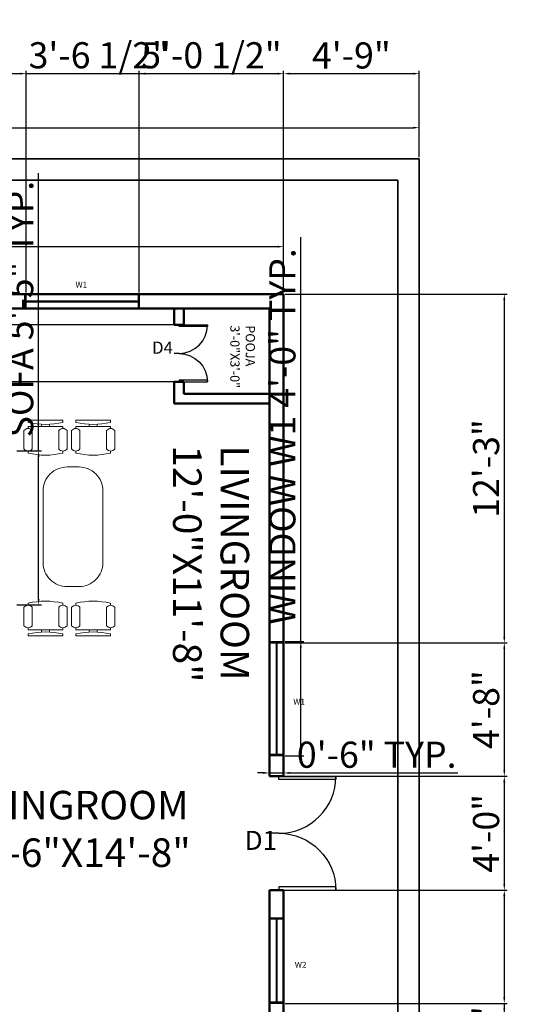
# Model space of a CAD drawing. Units: inches. Extents: x 2299 to 4423, y 1066 to 1805.
# Tile 3 of 7: x 2670 to 2884, y 1391 to 1805. Entities that reach past the tile are written whole.
import ezdxf

# ---------------------------------------------------------------- set-up
doc = ezdxf.new("R2010")
doc.units = ezdxf.units.IN
for name, color, linetype, lineweight in [('A-ANNO-DIMS', 2, 'Continuous', 18), ('A-ANNO-TEXT', 1, 'Continuous', 25), ('A-AREA-IDEN', 1, 'Continuous', 25), ('A-DOOR', 5, 'Continuous', 25), ('A-FURN', 8, 'Continuous', 18), ('A-GLAZ', 3, 'Continuous', 25), ('A-WALL', 7, 'Continuous', 50), ('C-PROP', 7, 'Continuous', 35)]:
    doc.layers.add(name, color=color, linetype=linetype, lineweight=lineweight)
doc.styles.get("Standard").update_dxf_attribs({"font": 'arial.ttf'})
doc.dimstyles.new('ISO-25', dxfattribs={"dimtxt": 11, "dimasz": 2.5, "dimexe": 1.25, "dimexo": 0.625, "dimtad": 1, "dimlunit": 4, "dimtxsty": 'Standard', "dimcen": 2.5, "dimadec": 0, "dimazin": 0, "dimtfac": 1, "dimtmove": 0, "dimatfit": 3, "dimfxl": 1, "dimarcsym": 0})

# ---------------------------------------------------------------- blocks, each defined once
blk = doc.blocks.new('*U2')
for p, q in [((0, 0), (0, -5)), ((30, 0), (30, -5))]:
    blk.add_line(p, q)
blk.add_lwpolyline([(0, 0), (0, 30), (1.75, 30), (1.75, 0)], close=True)
blk.add_arc((0, 0), 30, 0, 90)
blk = doc.blocks.new('Chair - Desk')
for p, q in [((-8.5, 0), (-8.5, -1)), ((-8.5, 0), (8.5, 0)), ((8.5, 0), (8.5, -1)), ((-8.5, -3), (-8.5, -4)), ((-8.5, -3), (8.5, -3)), ((-2, -3), (-2, -1.9355)), ((2, -1.9576), (2, -3)), ((8.5, -3), (8.5, -4)), ((-10.5, -5), (-10.5, -14)), ((-6.5, -14), (-6.5, -5)), ((6.5, -5), (6.5, -14)), ((10.5, -14), (10.5, -5)), ((-8.5, -15), (-8.5, -16)), ((8.5, -15), (8.5, -16))]:
    blk.add_line(p, q)
for centre, radius, start, end in [((-8.5, -6.5), 2.5, 36.8699, 143.1301), ((0, 34.625), 36.625, 256.5803, 283.4197), ((8.5, -6.5), 2.5, 36.8699, 143.1301), ((-8.5, -12.5), 2.5, 216.8699, 323.1301), ((8.5, -12.5), 2.5, 216.8699, 323.1301), ((0, 19.625), 36.625, 256.5803, 283.4197)]:
    blk.add_arc(centre, radius, start, end)
blk = doc.blocks.new('*D20')
at = {"layer": 'A-ANNO-DIMS', "color": 0, "lineweight": -2, "transparency": 16777216}
for p, q in [((2357.83, 1747.57), (2357.83, 1761.24)), ((2360.33, 1759.99), (2835.33, 1759.99)), ((2837.83, 1747.57), (2837.83, 1761.24))]:
    blk.add_line(p, q, dxfattribs=at)
at = {"layer": 'A-ANNO-DIMS', "color": 0, "transparency": 16777216}
for points in [[(2360.33, 1760.41), (2360.33, 1759.58), (2357.83, 1759.99)], [(2835.33, 1760.41), (2835.33, 1759.58), (2837.83, 1759.99)]]:
    blk.add_solid(points, dxfattribs=at)
at = {"layer": 'Defpoints', "color": 0, "transparency": 16777216}
for p in [(2837.83, 1759.99), (2357.83, 1746.95), (2837.83, 1746.95)]:
    blk.add_point(p, dxfattribs=at)
at = {"layer": 'A-ANNO-DIMS', "color": 0, "transparency": 16777216, "insert": (2597.83, 1766.23), "char_height": 11, "attachment_point": 5}
blk.add_mtext("40'", dxfattribs=at)
blk = doc.blocks.new('*D22')
at = {"layer": 'A-ANNO-DIMS', "color": 0, "lineweight": -2, "transparency": 16777216}
for p, q in [((2414.83, 1690.57), (2414.83, 1711.17)), ((2417.33, 1709.92), (2778.33, 1709.92)), ((2780.83, 1690.57), (2780.83, 1711.17))]:
    blk.add_line(p, q, dxfattribs=at)
at = {"layer": 'A-ANNO-DIMS', "color": 0, "transparency": 16777216}
for points in [[(2417.33, 1710.33), (2417.33, 1709.5), (2414.83, 1709.92)], [(2778.33, 1710.33), (2778.33, 1709.5), (2780.83, 1709.92)]]:
    blk.add_solid(points, dxfattribs=at)
at = {"layer": 'Defpoints', "color": 0, "transparency": 16777216}
for p in [(2780.83, 1709.92), (2414.83, 1689.95), (2780.83, 1689.95)]:
    blk.add_point(p, dxfattribs=at)
at = {"layer": 'A-ANNO-DIMS', "color": 0, "transparency": 16777216, "insert": (2597.83, 1716.16), "char_height": 11, "attachment_point": 5}
blk.add_mtext('30\'-6"', dxfattribs=at)
blk = doc.blocks.new('WIN-1200')
for p, q in [((0, 0), (0, 48.07)), ((0, 48.07), (6, 48.07)), ((0, 47.57), (6, 47.57)), ((2.8, 47.57), (2.8, 0.5)), ((3.2, 47.57), (3.2, 0.5)), ((6, 48.07), (6, 0)), ((6, 0.5), (0, 0.5)), ((6, 0), (0, 0))]:
    blk.add_line(p, q)
blk = doc.blocks.new('WIN-900')
for p, q in [((0, 6), (36.07, 6)), ((0, 0), (0, 6)), ((0.5, 0), (0.5, 6)), ((35.57, 6), (35.57, 0)), ((36.07, 6), (36.07, 0)), ((36.07, 0), (0, 0)), ((0.5, 3.2), (35.57, 3.2)), ((0.5, 2.8), (35.57, 2.8))]:
    blk.add_line(p, q)
blk = doc.blocks.new('*D38')
at = {"layer": 'A-ANNO-DIMS', "color": 0, "lineweight": -2, "transparency": 16777216}
for p, q in [((2788.04, 1543.64), (2788.04, 1713.9)), ((2781.46, 1543.64), (2789.29, 1543.64)), ((2788.04, 1498.07), (2788.04, 1541.14)), ((2781.46, 1495.57), (2789.29, 1495.57))]:
    blk.add_line(p, q, dxfattribs=at)
at = {"layer": 'A-ANNO-DIMS', "color": 0, "transparency": 16777216}
for points in [[(2787.63, 1541.14), (2788.46, 1541.14), (2788.04, 1543.64)], [(2787.63, 1498.07), (2788.46, 1498.07), (2788.04, 1495.57)]]:
    blk.add_solid(points, dxfattribs=at)
at = {"layer": 'Defpoints', "color": 0, "transparency": 16777216}
for p in [(2780.83, 1543.64), (2788.04, 1543.64), (2780.83, 1495.57)]:
    blk.add_point(p, dxfattribs=at)
at = {"layer": 'A-ANNO-DIMS', "color": 0, "transparency": 16777216, "insert": (2781.73, 1630.02), "char_height": 11, "attachment_point": 5, "rotation": 90}
blk.add_mtext('WINDOW W1 4\'-0" TYP.', dxfattribs=at)
blk = doc.blocks.new('*D39')
at = {"layer": 'A-ANNO-DIMS', "color": 0, "lineweight": -2, "transparency": 16777216}
for p, q in [((2774.83, 1494.94), (2774.83, 1487.1)), ((2780.83, 1494.94), (2780.83, 1487.1)), ((2772.33, 1488.35), (2769.83, 1488.35)), ((2774.83, 1488.35), (2780.83, 1488.35)), ((2783.33, 1488.35), (2854.13, 1488.35))]:
    blk.add_line(p, q, dxfattribs=at)
at = {"layer": 'A-ANNO-DIMS', "color": 0, "transparency": 16777216}
for points in [[(2772.33, 1488.77), (2772.33, 1487.94), (2774.83, 1488.35)], [(2783.33, 1488.77), (2783.33, 1487.94), (2780.83, 1488.35)]]:
    blk.add_solid(points, dxfattribs=at)
at = {"layer": 'Defpoints', "color": 0, "transparency": 16777216}
for p in [(2774.83, 1495.57), (2780.83, 1495.57), (2780.83, 1488.35)]:
    blk.add_point(p, dxfattribs=at)
at = {"layer": 'A-ANNO-DIMS', "color": 0, "transparency": 16777216, "insert": (2819.98, 1494.6), "char_height": 11, "attachment_point": 5}
blk.add_mtext('0\'-6" TYP.', dxfattribs=at)
blk = doc.blocks.new('*D52')
at = {"layer": 'A-ANNO-DIMS', "color": 0, "lineweight": -2, "transparency": 16777216}
for p, q in [((2677.79, 1623.96), (2677.79, 1740.82)), ((2668.68, 1623.96), (2679.04, 1623.96)), ((2677.79, 1561.58), (2677.79, 1621.46)), ((2668.68, 1559.08), (2679.04, 1559.08))]:
    blk.add_line(p, q, dxfattribs=at)
at = {"layer": 'A-ANNO-DIMS', "color": 0, "transparency": 16777216}
for points in [[(2677.37, 1621.46), (2678.21, 1621.46), (2677.79, 1623.96)], [(2677.37, 1561.58), (2678.21, 1561.58), (2677.79, 1559.08)]]:
    blk.add_solid(points, dxfattribs=at)
at = {"layer": 'Defpoints', "color": 0, "transparency": 16777216}
for p in [(2668.06, 1623.96), (2677.79, 1623.96), (2668.06, 1559.08)]:
    blk.add_point(p, dxfattribs=at)
at = {"layer": 'A-ANNO-DIMS', "color": 0, "transparency": 16777216, "insert": (2671.47, 1683.64), "char_height": 11, "attachment_point": 5, "rotation": 90}
blk.add_mtext('SOFA 5\'-5" TYP.', dxfattribs=at)
blk = doc.blocks.new('*D67')
at = {"layer": 'A-ANNO-DIMS', "color": 0, "lineweight": -2, "transparency": 16777216}
for p, q in [((2629.83, 1684.57), (2629.83, 1784)), ((2632.33, 1782.75), (2670.06, 1782.75)), ((2672.56, 1690.57), (2672.56, 1784)), ((2672.56, 1782.75), (2731.17, 1782.75))]:
    blk.add_line(p, q, dxfattribs=at)
at = {"layer": 'A-ANNO-DIMS', "color": 0, "transparency": 16777216}
for points in [[(2632.33, 1783.16), (2632.33, 1782.33), (2629.83, 1782.75)], [(2670.06, 1783.16), (2670.06, 1782.33), (2672.56, 1782.75)]]:
    blk.add_solid(points, dxfattribs=at)
at = {"layer": 'Defpoints', "color": 0, "transparency": 16777216}
for p in [(2672.56, 1782.75), (2672.56, 1689.95), (2629.83, 1683.95)]:
    blk.add_point(p, dxfattribs=at)
at = {"layer": 'A-ANNO-DIMS', "color": 0, "transparency": 16777216, "insert": (2703.11, 1789.06), "char_height": 11, "attachment_point": 5}
blk.add_mtext('3\'-6 1/2"', dxfattribs=at)
blk = doc.blocks.new('*D68')
at = {"layer": 'A-ANNO-DIMS', "color": 0, "lineweight": -2, "transparency": 16777216}
for p, q in [((2720.13, 1690.57), (2720.13, 1784)), ((2722.63, 1782.75), (2778.33, 1782.75)), ((2780.83, 1690.57), (2780.83, 1784))]:
    blk.add_line(p, q, dxfattribs=at)
at = {"layer": 'A-ANNO-DIMS', "color": 0, "transparency": 16777216}
for points in [[(2722.63, 1783.16), (2722.63, 1782.33), (2720.13, 1782.75)], [(2778.33, 1783.16), (2778.33, 1782.33), (2780.83, 1782.75)]]:
    blk.add_solid(points, dxfattribs=at)
at = {"layer": 'Defpoints', "color": 0, "transparency": 16777216}
for p in [(2780.83, 1782.75), (2720.13, 1689.95), (2780.83, 1689.95)]:
    blk.add_point(p, dxfattribs=at)
at = {"layer": 'A-ANNO-DIMS', "color": 0, "transparency": 16777216, "insert": (2750.48, 1789.06), "char_height": 11, "attachment_point": 5}
blk.add_mtext('5\'-0 1/2"', dxfattribs=at)
blk = doc.blocks.new('*D69')
at = {"layer": 'A-ANNO-DIMS', "color": 0, "lineweight": -2, "transparency": 16777216}
for p, q in [((2780.83, 1690.57), (2780.83, 1784)), ((2783.33, 1782.75), (2835.33, 1782.75)), ((2837.83, 1747.57), (2837.83, 1784))]:
    blk.add_line(p, q, dxfattribs=at)
at = {"layer": 'A-ANNO-DIMS', "color": 0, "transparency": 16777216}
for points in [[(2783.33, 1783.16), (2783.33, 1782.33), (2780.83, 1782.75)], [(2835.33, 1783.16), (2835.33, 1782.33), (2837.83, 1782.75)]]:
    blk.add_solid(points, dxfattribs=at)
at = {"layer": 'Defpoints', "color": 0, "transparency": 16777216}
for p in [(2837.83, 1782.75), (2837.83, 1746.95), (2780.83, 1689.95)]:
    blk.add_point(p, dxfattribs=at)
at = {"layer": 'A-ANNO-DIMS', "color": 0, "transparency": 16777216, "insert": (2809.33, 1788.99), "char_height": 11, "attachment_point": 5}
blk.add_mtext('4\'-9"', dxfattribs=at)
blk = doc.blocks.new('*D78')
at = {"layer": 'A-ANNO-DIMS', "color": 0, "lineweight": -2, "transparency": 16777216}
for p, q in [((2781.46, 1689.95), (2874.88, 1689.95)), ((2873.63, 1687.45), (2873.63, 1545.64)), ((2781.46, 1543.14), (2874.88, 1543.14))]:
    blk.add_line(p, q, dxfattribs=at)
at = {"layer": 'A-ANNO-DIMS', "color": 0, "transparency": 16777216}
for points in [[(2873.22, 1687.45), (2874.05, 1687.45), (2873.63, 1689.95)], [(2873.22, 1545.64), (2874.05, 1545.64), (2873.63, 1543.14)]]:
    blk.add_solid(points, dxfattribs=at)
at = {"layer": 'Defpoints', "color": 0, "transparency": 16777216}
for p in [(2780.83, 1689.95), (2780.83, 1543.14), (2873.63, 1543.14)]:
    blk.add_point(p, dxfattribs=at)
at = {"layer": 'A-ANNO-DIMS', "color": 0, "transparency": 16777216, "insert": (2867.39, 1616.54), "char_height": 11, "attachment_point": 5, "rotation": 90}
blk.add_mtext('12\'-3"', dxfattribs=at)
blk = doc.blocks.new('*D79')
at = {"layer": 'A-ANNO-DIMS', "color": 0, "lineweight": -2, "transparency": 16777216}
for p, q in [((2781.46, 1543.14), (2874.88, 1543.14)), ((2873.63, 1540.64), (2873.63, 1489.45)), ((2781.46, 1486.95), (2874.88, 1486.95))]:
    blk.add_line(p, q, dxfattribs=at)
at = {"layer": 'A-ANNO-DIMS', "color": 0, "transparency": 16777216}
for points in [[(2873.22, 1540.64), (2874.05, 1540.64), (2873.63, 1543.14)], [(2873.22, 1489.45), (2874.05, 1489.45), (2873.63, 1486.95)]]:
    blk.add_solid(points, dxfattribs=at)
at = {"layer": 'Defpoints', "color": 0, "transparency": 16777216}
for p in [(2780.83, 1543.14), (2780.83, 1486.95), (2873.63, 1486.95)]:
    blk.add_point(p, dxfattribs=at)
at = {"layer": 'A-ANNO-DIMS', "color": 0, "transparency": 16777216, "insert": (2867.39, 1515.04), "char_height": 11, "attachment_point": 5, "rotation": 90}
blk.add_mtext('4\'-8"', dxfattribs=at)
blk = doc.blocks.new('*D80')
at = {"layer": 'A-ANNO-DIMS', "color": 0, "lineweight": -2, "transparency": 16777216}
for p, q in [((2781.46, 1486.95), (2874.88, 1486.95)), ((2873.63, 1484.45), (2873.63, 1441.45)), ((2781.46, 1438.95), (2874.88, 1438.95))]:
    blk.add_line(p, q, dxfattribs=at)
at = {"layer": 'A-ANNO-DIMS', "color": 0, "transparency": 16777216}
for points in [[(2873.22, 1484.45), (2874.05, 1484.45), (2873.63, 1486.95)], [(2873.22, 1441.45), (2874.05, 1441.45), (2873.63, 1438.95)]]:
    blk.add_solid(points, dxfattribs=at)
at = {"layer": 'Defpoints', "color": 0, "transparency": 16777216}
for p in [(2780.83, 1486.95), (2780.83, 1438.95), (2873.63, 1438.95)]:
    blk.add_point(p, dxfattribs=at)
at = {"layer": 'A-ANNO-DIMS', "color": 0, "transparency": 16777216, "insert": (2867.39, 1462.95), "char_height": 11, "attachment_point": 5, "rotation": 90}
blk.add_mtext('4\'-0"', dxfattribs=at)
blk = doc.blocks.new('*D81')
at = {"layer": 'A-ANNO-DIMS', "color": 0, "lineweight": -2, "transparency": 16777216}
for p, q in [((2781.46, 1438.95), (2874.88, 1438.95)), ((2873.63, 1436.45), (2873.63, 1393.85)), ((2781.46, 1391.35), (2874.88, 1391.35)), ((2873.63, 1391.35), (2873.63, 1324.19))]:
    blk.add_line(p, q, dxfattribs=at)
at = {"layer": 'A-ANNO-DIMS', "color": 0, "transparency": 16777216}
for points in [[(2873.22, 1436.45), (2874.05, 1436.45), (2873.63, 1438.95)], [(2873.22, 1393.85), (2874.05, 1393.85), (2873.63, 1391.35)]]:
    blk.add_solid(points, dxfattribs=at)
at = {"layer": 'Defpoints', "color": 0, "transparency": 16777216}
for p in [(2780.83, 1438.95), (2780.83, 1391.35), (2873.63, 1391.35)]:
    blk.add_point(p, dxfattribs=at)
at = {"layer": 'A-ANNO-DIMS', "color": 0, "transparency": 16777216, "insert": (2867.32, 1356.52), "char_height": 11, "attachment_point": 5, "rotation": 90}
blk.add_mtext('3\'-11 1/2"', dxfattribs=at)
blk = doc.blocks.new('*D82')
at = {"layer": 'A-ANNO-DIMS', "color": 0, "lineweight": -2, "transparency": 16777216}
for p, q in [((2781.46, 1391.35), (2874.88, 1391.35)), ((2873.63, 1388.85), (2873.63, 1356.45)), ((2781.46, 1353.95), (2874.88, 1353.95)), ((2873.63, 1353.95), (2873.63, 1295.33))]:
    blk.add_line(p, q, dxfattribs=at)
at = {"layer": 'A-ANNO-DIMS', "color": 0, "transparency": 16777216}
for points in [[(2873.22, 1388.85), (2874.05, 1388.85), (2873.63, 1391.35)], [(2873.22, 1356.45), (2874.05, 1356.45), (2873.63, 1353.95)]]:
    blk.add_solid(points, dxfattribs=at)
at = {"layer": 'Defpoints', "color": 0, "transparency": 16777216}
for p in [(2780.83, 1391.35), (2780.83, 1353.95), (2873.63, 1353.95)]:
    blk.add_point(p, dxfattribs=at)
at = {"layer": 'A-ANNO-DIMS', "color": 0, "transparency": 16777216, "insert": (2867.32, 1323.39), "char_height": 11, "attachment_point": 5, "rotation": 90}
blk.add_mtext('3\'-1 1/2"', dxfattribs=at)
blk = doc.blocks.new('*D89')
at = {"layer": 'A-ANNO-DIMS', "color": 0, "lineweight": -2, "transparency": 16777216}
for p, q in [((2738.21, 1676.95), (2320.78, 1676.95)), ((2322.03, 1674.45), (2322.03, 1655.45)), ((2738.21, 1652.95), (2320.78, 1652.95)), ((2322.03, 1652.95), (2322.03, 1619.77))]:
    blk.add_line(p, q, dxfattribs=at)
at = {"layer": 'A-ANNO-DIMS', "color": 0, "transparency": 16777216}
for points in [[(2321.62, 1674.45), (2322.45, 1674.45), (2322.03, 1676.95)], [(2321.62, 1655.45), (2322.45, 1655.45), (2322.03, 1652.95)]]:
    blk.add_solid(points, dxfattribs=at)
at = {"layer": 'Defpoints', "color": 0, "transparency": 16777216}
for p in [(2738.83, 1676.95), (2322.03, 1652.95), (2738.83, 1652.95)]:
    blk.add_point(p, dxfattribs=at)
at = {"layer": 'A-ANNO-DIMS', "color": 0, "transparency": 16777216, "insert": (2315.79, 1635.11), "char_height": 11, "attachment_point": 5, "rotation": 90}
blk.add_mtext('2\'-0"', dxfattribs=at)

msp = doc.modelspace()

# ---------------------------------------------------------------- linework, layer by layer
at = {"layer": 'A-FURN'}
msp.add_lwpolyline([(2679.689, 1607.089, -0.4142136), (2689.759, 1617.159), (2694.794, 1617.159, -0.4142136), (2704.864, 1607.089), (2704.864, 1576.879, -0.4142136), (2694.794, 1566.809), (2689.759, 1566.809, -0.4142136), (2679.689, 1576.879)], format="xyb", close=True, dxfattribs=at)
at = {"layer": 'A-WALL'}
for p, q in [((2414.834, 1689.945), (2780.834, 1689.945)), ((2780.834, 1689.945), (2780.834, 1486.945)), ((2634.834, 1683.945), (2774.834, 1683.945)), ((2734.834, 1683.945), (2734.834, 1676.945)), ((2738.834, 1683.945), (2738.834, 1676.945)), ((2774.834, 1683.945), (2774.834, 1534.945)), ((2734.834, 1676.945), (2738.834, 1676.945)), ((2738.834, 1652.945), (2734.834, 1652.945)), ((2734.834, 1652.945), (2734.834, 1643.945)), ((2738.834, 1647.945), (2738.834, 1652.945)), ((2738.834, 1652.945), (2738.834, 1647.945)), ((2738.834, 1647.945), (2774.834, 1647.945)), ((2734.834, 1643.945), (2774.834, 1643.945)), ((2774.834, 1534.945), (2774.834, 1486.945)), ((2780.834, 1486.945), (2774.834, 1486.945)), ((2774.834, 1438.945), (2780.834, 1438.945)), ((2774.834, 1438.945), (2774.834, 1358.945)), ((2780.834, 1438.945), (2780.834, 1353.945))]:
    msp.add_line(p, q, dxfattribs=at)
at = {"layer": 'C-PROP'}
for p, q in [((2357.834, 1746.945), (2837.834, 1746.945)), ((2837.834, 1746.945), (2837.834, 1170.945)), ((2366.834, 1737.945), (2828.834, 1737.945)), ((2828.834, 1737.945), (2828.834, 1179.945))]:
    msp.add_line(p, q, dxfattribs=at)

# ---------------------------------------------------------------- block references
at = {"layer": 'A-DOOR', "rotation": 270}
for p, xscale, yscale, zscale in [((2736.834, 1676.945), 0.4000000000000031, 0.4000000000000031, 0.4000000000000031), ((2736.834, 1652.945), -0.4000000000000031, 0.4000000000000031, 0.4000000000000031), ((2778.832, 1486.92), 0.7995697346464069, 0.7995697346464069, 0.7995697346464069), ((2778.832, 1438.945), -0.7995697346464069, 0.7995697346464069, 0.7995697346464069)]:
    msp.add_blockref('*U2', p, dxfattribs=dict(at, xscale=xscale, yscale=yscale, zscale=zscale))
at = {"layer": 'A-FURN', "xscale": 0.8626440446238717, "yscale": 0.8626440446238717, "zscale": 0.8626440446238717}
for p in [(2680.69, 1636.808), (2700.747, 1636.808)]:
    msp.add_blockref('Chair - Desk', p, dxfattribs=at)
at = {"layer": 'A-FURN', "xscale": -0.8626440446238717, "yscale": 0.8626440446238717, "zscale": 0.8626440446238717, "rotation": 180}
for p in [(2680.69, 1546.004), (2700.747, 1546.004)]:
    msp.add_blockref('Chair - Desk', p, dxfattribs=at)
at = {"layer": 'A-GLAZ'}
for name, p, rotation in [('WIN-1200', (2720.127, 1683.945), 90.0000000000004), ('WIN-900', (2774.833, 1427.42), 269.9999999999989)]:
    msp.add_blockref(name, p, dxfattribs=dict(at, rotation=rotation))
msp.add_blockref('WIN-1200', (2774.834, 1495.565), dxfattribs=at)

# ---------------------------------------------------------------- texts
at = {"layer": 'A-ANNO-TEXT', "char_height": 2.5, "attachment_point": 1}
for s, insert in [('W1', (2693.301, 1695.161)), ('W1', (2784.895, 1519.601)), ('W2', (2785.537, 1408.822))]:
    msp.add_mtext(s, dxfattribs=dict(at, insert=insert))
at = {"layer": 'A-ANNO-TEXT', "attachment_point": 1}
for s, width, gutter_width, insert, char_height in [('D4', 0.71689, 8.065, (2725.507, 1669.979), 5.1613), ('D1', 1.11117, 12.5, (2764.486, 1463.973), 8)]:
    msp.add_mtext_dynamic_manual_height_columns(s, width=width, gutter_width=gutter_width, heights=[0], dxfattribs=dict(at, insert=insert, char_height=char_height))
at = {"layer": 'A-AREA-IDEN', "attachment_point": 1, "rotation": 270}
for s, width, gutter_width, insert, char_height in [('POOJA\\P3\'-0"X3\'-0"', 4.35314, 19.417, (2768.761, 1676.808), 3.88333), ('LIVINGROOM\\P12\'-0"X11\'-8"', 9.28623, 12.5, (2766.318, 1626.268), 12)]:
    msp.add_mtext_dynamic_manual_height_columns(s, width=width, gutter_width=gutter_width, heights=[0], dxfattribs=dict(at, insert=insert, char_height=char_height))
at = {"layer": 'A-AREA-IDEN', "insert": (2641.889, 1480.805), "char_height": 12, "attachment_point": 1}
msp.add_mtext_dynamic_manual_height_columns('LIVINGROOM\\P17\'-6"X14\'-8"', width=12, gutter_width=12.5, heights=[0], dxfattribs=at)

# ---------------------------------------------------------------- dimensions: what is measured, and where the dimension line sits
at = {"layer": 'A-ANNO-DIMS'}
for base, p1, p2, override, picture, middle in [((2672.556, 1782.745), (2629.834, 1683.945), (2672.556, 1689.945), {"dimdec": 1, "dimlfac": 1, "dimrnd": 0, "dimzin": 1, "dimdsep": 46, "dimlunit": 4, "dimfrac": 2}, '*D67', (2703.114, 1789.062)), ((2780.834, 1782.745), (2720.127, 1689.945), (2780.834, 1689.945), {"dimdec": 1, "dimlfac": 1, "dimrnd": 0, "dimzin": 1, "dimdsep": 46, "dimlunit": 4, "dimfrac": 2}, '*D68', (2750.48, 1789.058)), ((2837.834, 1782.745), (2780.834, 1689.945), (2837.834, 1746.945), {"dimdec": 1, "dimlfac": 1, "dimrnd": 0, "dimzin": 1, "dimdsep": 46, "dimlunit": 4, "dimfrac": 2}, '*D69', (2809.334, 1788.987)), ((2837.834, 1759.993), (2357.834, 1746.945), (2837.834, 1746.945), {"dimclrd": 0, "dimclre": 0, "dimclrt": 0}, '*D20', (2597.834, 1766.235)), ((2780.834, 1709.917), (2414.834, 1689.945), (2780.834, 1689.945), {"dimclrd": 0, "dimclre": 0, "dimclrt": 0}, '*D22', (2597.834, 1716.162))]:
    dim = msp.add_linear_dim(base=base, p1=p1, p2=p2, dimstyle='ISO-25', override=override, dxfattribs=at)
    dim.commit()
    dim.dimension.update_dxf_attribs({"geometry": picture, "text_midpoint": middle})
for base, p1, p2, text, picture, middle in [((2677.789, 1623.965), (2668.057, 1559.081), (2668.057, 1623.965), 'SOFA <> TYP.', '*D52', (2671.473, 1683.643)), ((2788.044, 1543.636), (2780.834, 1495.565), (2780.834, 1543.636), 'WINDOW W1 <> TYP.', '*D38', (2781.728, 1630.019))]:
    dim = msp.add_linear_dim(base=base, p1=p1, p2=p2, angle=90, text=text, dimstyle='ISO-25', override={"dimdec": 1, "dimrnd": 0, "dimzin": 1, "dimlunit": 4, "dimfrac": 2}, dxfattribs=at)
    dim.commit()
    dim.dimension.update_dxf_attribs({"geometry": picture, "text_midpoint": middle})
for base, p1, p2, picture, middle in [((2873.634, 1543.136), (2780.834, 1689.945), (2780.834, 1543.136), '*D78', (2867.389, 1616.541)), ((2322.034, 1652.945), (2738.834, 1676.945), (2738.834, 1652.945), '*D89', (2315.792, 1635.106)), ((2873.634, 1486.945), (2780.834, 1543.136), (2780.834, 1486.945), '*D79', (2867.392, 1515.041)), ((2873.634, 1438.945), (2780.834, 1486.945), (2780.834, 1438.945), '*D80', (2867.392, 1462.945)), ((2873.634, 1391.349), (2780.834, 1438.945), (2780.834, 1391.349), '*D81', (2867.317, 1356.518)), ((2873.634, 1353.945), (2780.834, 1391.349), (2780.834, 1353.945), '*D82', (2867.317, 1323.388))]:
    dim = msp.add_linear_dim(base=base, p1=p1, p2=p2, angle=90, dimstyle='ISO-25', override={"dimdec": 1, "dimlfac": 1, "dimrnd": 0, "dimzin": 1, "dimdsep": 46, "dimlunit": 4, "dimfrac": 2}, dxfattribs=at)
    dim.commit()
    dim.dimension.update_dxf_attribs({"geometry": picture, "text_midpoint": middle})
dim = msp.add_linear_dim(base=(2780.834, 1488.355), p1=(2774.834, 1495.565), p2=(2780.834, 1495.565), text='<> TYP.', dimstyle='ISO-25', override={"dimdec": 1, "dimrnd": 0, "dimzin": 1, "dimlunit": 4, "dimfrac": 2}, dxfattribs=at)
dim.commit()
dim.dimension.update_dxf_attribs({"geometry": '*D39', "text_midpoint": (2819.984, 1494.596)})

doc.saveas('drawing.dxf')
